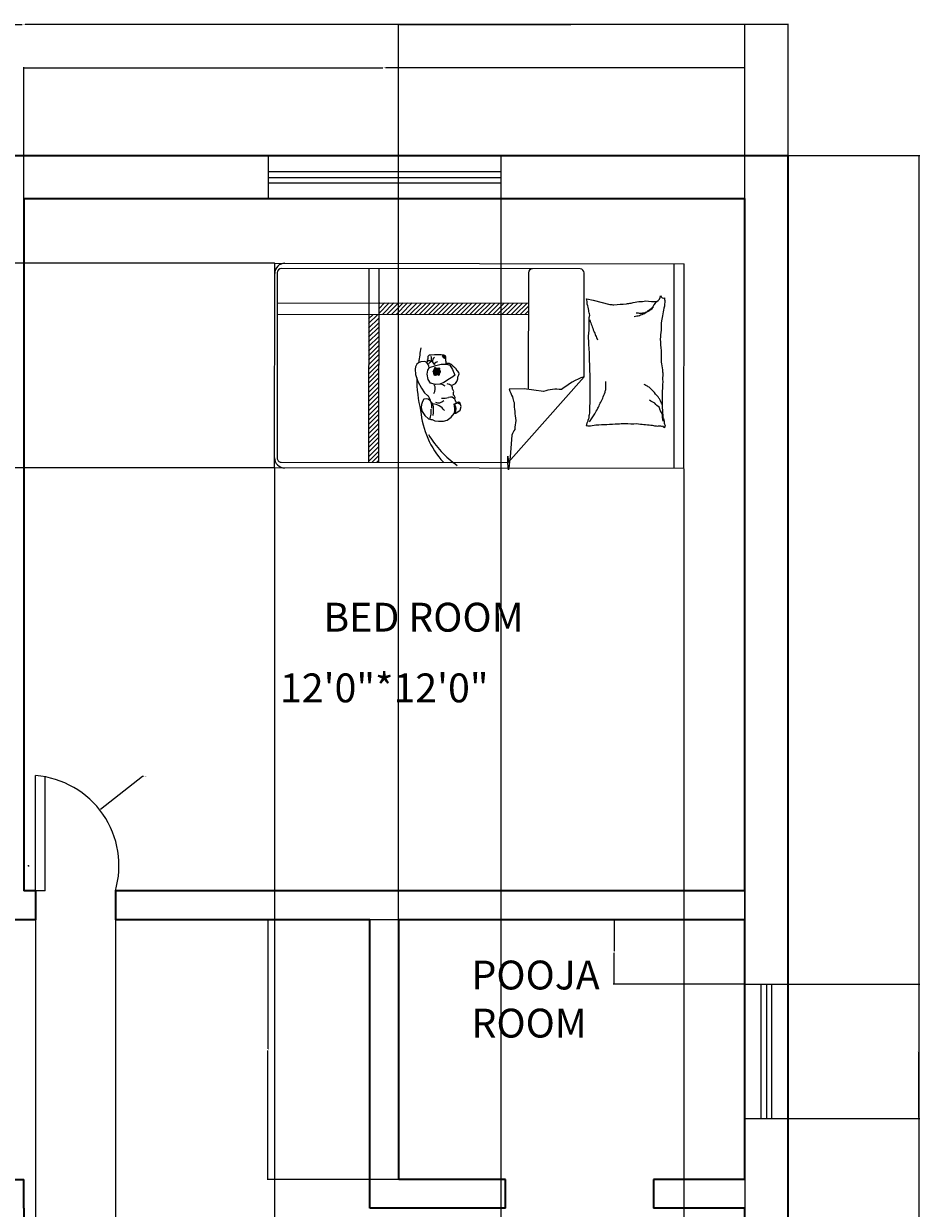
# Model space of a CAD drawing. Units: inches. Extents: x -17 to 1735, y -531 to 60.
# Tile 4 of 27: x 170 to 357, y -187 to 60. Entities that reach past the tile are written whole.
import ezdxf

# ---------------------------------------------------------------- set-up
doc = ezdxf.new("R2010")
doc.units = ezdxf.units.IN
doc.header["$MEASUREMENT"] = 0
for name, color, linetype, lineweight in [('A-ANNO-DIMS', 2, 'Continuous', 18), ('A-AREA-IDEN', 7, 'Continuous', 25), ('A-DOOR', 4, 'Continuous', 18), ('A-GLAZ', 4, 'Continuous', 18), ('A-WALL', 7, 'Continuous', 35)]:
    doc.layers.add(name, color=color, linetype=linetype, lineweight=lineweight)
doc.layers.add('A-FURN', color=242, linetype='Continuous', lineweight=18, true_color=0xcd2027)
doc.layers.add('A-FURN-PATT', color=242, linetype='Continuous', lineweight=13, true_color=0xcd2027)
doc.styles.get("Standard").update_dxf_attribs({"font": 'arial.ttf'})
doc.dimstyles.get("Standard").update_dxf_attribs({"dimtxt": 0.18, "dimasz": 0.18, "dimexe": 0.18, "dimexo": 0.0625, "dimgap": 0.09, "dimtad": 0, "dimtih": 1, "dimtoh": 1, "dimdec": 4, "dimzin": 0, "dimdsep": 46, "dimtxsty": 'Standard', "dimcen": 0.09, "dimadec": 0, "dimazin": 0, "dimtfac": 1, "dimtdec": 4, "dimtofl": 0, "dimtmove": 0, "dimatfit": 3, "dimfxl": 1, "dimtolj": 1, "dimtzin": 0, "dimarcsym": 0})
pattern_1 = [(314.93283, (734.16654, -492.2216), (0.082070428, 0.081878224), [])]

# ---------------------------------------------------------------- blocks, each defined once
blk = doc.blocks.new('WIN-FRAME-48IN')
for p, q in [((3.31, 48.33), (3.31, 0)), ((5.59, 0), (5.59, 48.33))]:
    blk.add_line(p, q)
blk.add_lwpolyline([(0, 48.33), (9, 48.33), (9, 0), (0, 0)], close=True)
blk = doc.blocks.new('*D9')
at = {"layer": 'A-ANNO-DIMS', "color": 0, "lineweight": -2, "transparency": 16777216}
for p, q in [((11.06, 32.29), (11.06, 59.62)), ((11.24, 59.44), (169.77, 59.44)), ((328.88, 59.44), (170.35, 59.44)), ((329.06, 32.29), (329.06, 59.62))]:
    blk.add_line(p, q, dxfattribs=at)
at = {"layer": 'A-ANNO-DIMS', "color": 0, "transparency": 16777216}
for points in [[(11.24, 59.47), (11.24, 59.41), (11.06, 59.44)], [(328.88, 59.47), (328.88, 59.41), (329.06, 59.44)]]:
    blk.add_solid(points, dxfattribs=at)
at = {"layer": 'Defpoints', "color": 0, "transparency": 16777216}
for p in [(329.06, 59.44), (11.06, 32.23), (329.06, 32.23)]:
    blk.add_point(p, dxfattribs=at)
at = {"layer": 'A-ANNO-DIMS', "color": 0, "transparency": 16777216, "insert": (170.06, 59.44), "char_height": 0.18, "attachment_point": 5}
blk.add_mtext('\\A1;318', dxfattribs=at)
blk = doc.blocks.new('*D10')
at = {"layer": 'A-ANNO-DIMS', "color": 0, "lineweight": -2, "transparency": 16777216}
for p, q in [((329.12, 32.23), (356.44, 32.23)), ((356.26, 32.05), (356.26, -235.74)), ((356.26, -503.9), (356.26, -236.11)), ((329.12, -504.08), (356.44, -504.08))]:
    blk.add_line(p, q, dxfattribs=at)
at = {"layer": 'A-ANNO-DIMS', "color": 0, "transparency": 16777216}
for points in [[(356.23, 32.05), (356.29, 32.05), (356.26, 32.23)], [(356.23, -503.9), (356.29, -503.9), (356.26, -504.08)]]:
    blk.add_solid(points, dxfattribs=at)
at = {"layer": 'Defpoints', "color": 0, "transparency": 16777216}
for p in [(329.06, 32.23), (329.06, -504.08), (356.26, -504.08)]:
    blk.add_point(p, dxfattribs=at)
at = {"layer": 'A-ANNO-DIMS', "color": 0, "transparency": 16777216, "insert": (356.26, -235.92), "char_height": 0.18, "attachment_point": 5}
blk.add_mtext('\\A1;536.3', dxfattribs=at)
blk = doc.blocks.new('*D12')
at = {"layer": 'A-ANNO-DIMS', "color": 0, "lineweight": -2, "transparency": 16777216}
for p, q in [((269.33, 23.18), (269.33, -531.46)), ((320.06, 23.17), (320.06, -531.46)), ((269.51, -531.28), (294.3, -531.28)), ((319.88, -531.28), (295.09, -531.28))]:
    blk.add_line(p, q, dxfattribs=at)
at = {"layer": 'A-ANNO-DIMS', "color": 0, "transparency": 16777216}
for points in [[(269.51, -531.25), (269.51, -531.31), (269.33, -531.28)], [(319.88, -531.25), (319.88, -531.31), (320.06, -531.28)]]:
    blk.add_solid(points, dxfattribs=at)
at = {"layer": 'Defpoints', "color": 0, "transparency": 16777216}
for p in [(269.33, 23.24), (320.06, 23.23), (320.06, -531.28)]:
    blk.add_point(p, dxfattribs=at)
at = {"layer": 'A-ANNO-DIMS', "color": 0, "transparency": 16777216, "insert": (294.7, -531.28), "char_height": 0.18, "attachment_point": 5}
blk.add_mtext('\\A1;50.73', dxfattribs=at)
blk = doc.blocks.new('*D18')
at = {"layer": 'A-ANNO-DIMS', "color": 0, "lineweight": -2, "transparency": 16777216}
for p, q in [((320, -126.77), (292.68, -126.77)), ((292.86, -126.95), (292.86, -133.29)), ((292.86, -139.99), (292.86, -133.65)), ((320, -140.17), (292.68, -140.17))]:
    blk.add_line(p, q, dxfattribs=at)
at = {"layer": 'A-ANNO-DIMS', "color": 0, "transparency": 16777216}
for points in [[(292.83, -126.95), (292.89, -126.95), (292.86, -126.77)], [(292.83, -139.99), (292.89, -139.99), (292.86, -140.17)]]:
    blk.add_solid(points, dxfattribs=at)
at = {"layer": 'Defpoints', "color": 0, "transparency": 16777216}
for p in [(292.86, -126.77), (320.06, -126.77), (320.06, -140.17)]:
    blk.add_point(p, dxfattribs=at)
at = {"layer": 'A-ANNO-DIMS', "color": 0, "transparency": 16777216, "insert": (292.86, -133.47), "char_height": 0.18, "attachment_point": 5}
blk.add_mtext('\\A1;13.4', dxfattribs=at)
blk = doc.blocks.new('*D19')
at = {"layer": 'A-ANNO-DIMS', "color": 0, "lineweight": -2, "transparency": 16777216}
for p, q in [((320.12, -140.17), (356.44, -140.17)), ((356.26, -140.35), (356.26, -153.94)), ((356.26, -167.9), (356.26, -154.31)), ((320.12, -168.08), (356.44, -168.08))]:
    blk.add_line(p, q, dxfattribs=at)
at = {"layer": 'A-ANNO-DIMS', "color": 0, "transparency": 16777216}
for points in [[(356.23, -140.35), (356.29, -140.35), (356.26, -140.17)], [(356.23, -167.9), (356.29, -167.9), (356.26, -168.08)]]:
    blk.add_solid(points, dxfattribs=at)
at = {"layer": 'Defpoints', "color": 0, "transparency": 16777216}
for p in [(320.06, -140.17), (320.06, -168.08), (356.26, -168.08)]:
    blk.add_point(p, dxfattribs=at)
at = {"layer": 'A-ANNO-DIMS', "color": 0, "transparency": 16777216, "insert": (356.26, -154.12), "char_height": 0.18, "attachment_point": 5}
blk.add_mtext('\\A1;27.91', dxfattribs=at)
blk = doc.blocks.new('*D25')
at = {"layer": 'A-ANNO-DIMS', "color": 0, "lineweight": -2, "transparency": 16777216}
for p, q in [((248.06, -126.71), (248.06, 59.62)), ((248.24, 59.44), (283.84, 59.44)), ((319.88, 59.44), (284.28, 59.44)), ((320.06, -126.71), (320.06, 59.62))]:
    blk.add_line(p, q, dxfattribs=at)
at = {"layer": 'A-ANNO-DIMS', "color": 0, "transparency": 16777216}
for points in [[(248.24, 59.47), (248.24, 59.41), (248.06, 59.44)], [(319.88, 59.47), (319.88, 59.41), (320.06, 59.44)]]:
    blk.add_solid(points, dxfattribs=at)
at = {"layer": 'Defpoints', "color": 0, "transparency": 16777216}
for p in [(320.06, 59.44), (248.06, -126.77), (320.06, -126.77)]:
    blk.add_point(p, dxfattribs=at)
at = {"layer": 'A-ANNO-DIMS', "color": 0, "transparency": 16777216, "insert": (284.06, 59.44), "char_height": 0.18, "attachment_point": 5}
blk.add_mtext('\\A1;72', dxfattribs=at)
blk = doc.blocks.new('*D26')
at = {"layer": 'A-ANNO-DIMS', "color": 0, "lineweight": -2, "transparency": 16777216}
for p, q in [((248, -126.77), (220.68, -126.77)), ((220.86, -126.95), (220.86, -153.59)), ((220.86, -180.59), (220.86, -153.95)), ((248, -180.77), (220.68, -180.77))]:
    blk.add_line(p, q, dxfattribs=at)
at = {"layer": 'A-ANNO-DIMS', "color": 0, "transparency": 16777216}
for points in [[(220.83, -126.95), (220.89, -126.95), (220.86, -126.77)], [(220.83, -180.59), (220.89, -180.59), (220.86, -180.77)]]:
    blk.add_solid(points, dxfattribs=at)
at = {"layer": 'Defpoints', "color": 0, "transparency": 16777216}
for p in [(220.86, -126.77), (248.06, -126.77), (248.06, -180.77)]:
    blk.add_point(p, dxfattribs=at)
at = {"layer": 'A-ANNO-DIMS', "color": 0, "transparency": 16777216, "insert": (220.86, -153.77), "char_height": 0.18, "attachment_point": 5}
blk.add_mtext('\\A1;54', dxfattribs=at)
blk = doc.blocks.new('*D31')
at = {"layer": 'A-ANNO-DIMS', "color": 0, "lineweight": -2, "transparency": 16777216}
for p, q in [((172.55, -126.83), (172.55, -531.46)), ((189.13, -126.83), (189.13, -531.46)), ((172.73, -531.28), (180.46, -531.28)), ((188.95, -531.28), (181.23, -531.28))]:
    blk.add_line(p, q, dxfattribs=at)
at = {"layer": 'A-ANNO-DIMS', "color": 0, "transparency": 16777216}
for points in [[(172.73, -531.25), (172.73, -531.31), (172.55, -531.28)], [(188.95, -531.25), (188.95, -531.31), (189.13, -531.28)]]:
    blk.add_solid(points, dxfattribs=at)
at = {"layer": 'Defpoints', "color": 0, "transparency": 16777216}
for p in [(172.55, -126.77), (189.13, -126.77), (189.13, -531.28)]:
    blk.add_point(p, dxfattribs=at)
at = {"layer": 'A-ANNO-DIMS', "color": 0, "transparency": 16777216, "insert": (180.84, -531.28), "char_height": 0.18, "attachment_point": 5}
blk.add_mtext('\\A1;16.58', dxfattribs=at)
blk = doc.blocks.new('*D37')
at = {"layer": 'A-ANNO-DIMS', "color": 0, "lineweight": -2, "transparency": 16777216}
for p, q in [((222.24, -32.84), (222.24, -531.46)), ((307.4, -32.94), (307.4, -531.46)), ((222.42, -531.28), (264.43, -531.28)), ((307.22, -531.28), (265.21, -531.28))]:
    blk.add_line(p, q, dxfattribs=at)
at = {"layer": 'A-ANNO-DIMS', "color": 0, "transparency": 16777216}
for points in [[(222.42, -531.25), (222.42, -531.31), (222.24, -531.28)], [(307.22, -531.25), (307.22, -531.31), (307.4, -531.28)]]:
    blk.add_solid(points, dxfattribs=at)
at = {"layer": 'Defpoints', "color": 0, "transparency": 16777216}
for p in [(222.24, -32.78), (307.4, -32.88), (307.4, -531.28)]:
    blk.add_point(p, dxfattribs=at)
at = {"layer": 'A-ANNO-DIMS', "color": 0, "transparency": 16777216, "insert": (264.82, -531.28), "char_height": 0.18, "attachment_point": 5}
blk.add_mtext('\\A1;85.16', dxfattribs=at)
blk = doc.blocks.new('*D38')
at = {"layer": 'A-ANNO-DIMS', "color": 0, "lineweight": -2, "transparency": 16777216}
for p, q in [((222.23, 9.8), (-16.4, 9.8)), ((-16.22, 9.62), (-16.22, -11.31)), ((-16.22, -32.6), (-16.22, -11.67)), ((222.18, -32.78), (-16.4, -32.78))]:
    blk.add_line(p, q, dxfattribs=at)
at = {"layer": 'A-ANNO-DIMS', "color": 0, "transparency": 16777216}
for points in [[(-16.25, 9.62), (-16.19, 9.62), (-16.22, 9.8)], [(-16.25, -32.6), (-16.19, -32.6), (-16.22, -32.78)]]:
    blk.add_solid(points, dxfattribs=at)
at = {"layer": 'Defpoints', "color": 0, "transparency": 16777216}
for p in [(222.29, 9.8), (-16.22, -32.78), (222.24, -32.78)]:
    blk.add_point(p, dxfattribs=at)
at = {"layer": 'A-ANNO-DIMS', "color": 0, "transparency": 16777216, "insert": (-16.22, -11.49), "char_height": 0.18, "attachment_point": 5}
blk.add_mtext('\\A1;42.58', dxfattribs=at)
blk = doc.blocks.new('*D43')
at = {"layer": 'A-ANNO-DIMS', "color": 0, "lineweight": -2, "transparency": 16777216}
for p, q in [((170.06, 23.29), (170.06, 50.61)), ((170.24, 50.43), (244.78, 50.43)), ((319.88, 50.43), (245.34, 50.43)), ((320.06, 23.29), (320.06, 50.61))]:
    blk.add_line(p, q, dxfattribs=at)
at = {"layer": 'A-ANNO-DIMS', "color": 0, "transparency": 16777216}
for points in [[(170.24, 50.46), (170.24, 50.4), (170.06, 50.43)], [(319.88, 50.46), (319.88, 50.4), (320.06, 50.43)]]:
    blk.add_solid(points, dxfattribs=at)
at = {"layer": 'Defpoints', "color": 0, "transparency": 16777216}
for p in [(320.06, 50.43), (170.06, 23.23), (320.06, 23.23)]:
    blk.add_point(p, dxfattribs=at)
at = {"layer": 'A-ANNO-DIMS', "color": 0, "transparency": 16777216, "insert": (245.06, 50.43), "char_height": 0.18, "attachment_point": 5}
blk.add_mtext('\\A1;150', dxfattribs=at)
blk = doc.blocks.new('*D54')
at = {"layer": 'A-ANNO-DIMS', "color": 0, "lineweight": -2, "transparency": 16777216}
for p, q in [((194.79, -96.99), (186.04, -103.83)), ((194.97, -96.99), (194.79, -96.99)), ((170.99, -115.51), (171.17, -115.51)), ((171.08, -115.6), (171.08, -115.42))]:
    blk.add_line(p, q, dxfattribs=at)
at = {"layer": 'A-ANNO-DIMS', "color": 0, "transparency": 16777216}
blk.add_solid([(186.02, -103.8), (186.06, -103.85), (185.9, -103.94)], dxfattribs=at)
at = {"layer": 'Defpoints', "color": 0, "transparency": 16777216}
for p in [(185.9, -103.94), (171.08, -115.51)]:
    blk.add_point(p, dxfattribs=at)
at = {"layer": 'A-ANNO-DIMS', "color": 0, "transparency": 16777216, "insert": (195.38, -96.99), "char_height": 0.18, "attachment_point": 5}
blk.add_mtext('\\A1;R18.8', dxfattribs=at)

msp = doc.modelspace()

# ---------------------------------------------------------------- hatches: boundary and pattern name
at = {"layer": 'A-FURN-PATT'}
h = msp.add_hatch(dxfattribs=at)
h.set_pattern_fill('ANSI31', color=256, scale=0.21291, angle=-90.06717, style=0)
h.set_pattern_definition([(44.9328, (336.72006, -40.7893), (0.477435, -0.4785558), [])])
h.paths.add_polyline_path([(243.9098, 1.5357), (243.907, -0.8463), (275.0288, -0.8828), (275.0316, 1.4992)])
h.paths.add_polyline_path([(241.8205, -0.8439), (241.7845, -31.5931), (243.871, -31.5955), (243.907, -0.8463)])
h = msp.add_hatch(dxfattribs=at)
h.set_pattern_fill('ANSI31', color=256, scale=0.927434, angle=-90.06717, style=0)
h.set_pattern_definition(pattern_1)
h.paths.add_polyline_path([(257.8751, -9.9217), (257.8615, -9.709), (257.7919, -9.5225), (257.6134, -9.3824), (257.4737, -9.3201), (257.1071, -9.2829, 0.47935676)])
h = msp.add_hatch(dxfattribs=at)
h.set_pattern_fill('ANSI31', color=256, scale=0.927434, angle=-90.06717, style=0)
h.set_pattern_definition(pattern_1)
h.paths.add_polyline_path([(255.3459, -12.9354), (255.3281, -13.1639), (255.4098, -13.3866), (255.5619, -13.5157), (255.7375, -13.5159), (255.9894, -13.399), (256.1769, -13.3582), (256.2646, -13.4286), (256.3816, -13.4873), (256.5222, -13.4289), (256.5458, -13.3176), (256.5518, -13.1887), (256.6047, -13.0189), (256.7455, -12.8023), (256.769, -12.7437), (256.6229, -12.4916), (256.582, -12.3802), (256.6115, -12.2045), (256.6292, -12.0815), (256.5181, -11.9642), (256.4009, -12.005), (256.3013, -12.1221), (256.0846, -12.0984), (255.7042, -11.9456), (255.5227, -11.9806), (255.4991, -12.1036), (255.4756, -12.1973), (255.376, -12.2733), (255.3817, -12.3671), (255.3288, -12.5252), (255.2233, -12.6364), (255.1705, -12.6949), (255.2583, -12.7654)])

# ---------------------------------------------------------------- linework, layer by layer
at = {"layer": 'A-DOOR'}
for p, q in [((172.5508, -120.7685), (172.5508, -96.7685)), ((174.5508, -120.7685), (174.5508, -97.0339)), ((174.5508, -120.7685), (172.5508, -120.7685))]:
    msp.add_line(p, q, dxfattribs=at)
msp.add_arc((171.0813, -115.5103), 18.7993, 343.75767, 85.516486, dxfattribs=at)
at = {"layer": 'A-FURN'}
for p, q in [((222.238, -32.7807), (222.2879, 9.8012)), ((222.2879, 9.8012), (307.4519, 9.7014)), ((222.8038, 7.8496), (222.7586, -30.7191)), ((285.7962, 8.6274), (223.6564, 8.7003)), ((241.8317, 8.679), (241.7845, -31.5931)), ((243.9182, 8.6765), (243.871, -31.5955)), ((275.039, 7.7884), (275.0106, -16.4244)), ((286.6215, -13.8065), (286.6468, 7.7748)), ((286.6215, -13.8065), (270.8545, -31.6271)), ((223.6092, -31.5717), (270.8545, -31.6271)), ((307.402, -32.8805), (222.238, -32.7807))]:
    msp.add_line(p, q, dxfattribs=at)
for points in [[(305.3228, 9.7039), (305.2729, -32.878)], [(307.402, -32.8805), (307.4519, 9.7014)], [(222.7964, 1.5604), (275.0316, 1.4992)], [(222.7936, -0.8216), (275.0288, -0.8828)], [(256.7756, -9.2714), (256.2062, -9.2442), (255.544, -9.2832), (254.8421, -9.3089), (254.6302, -9.3351), (254.3786, -9.3481), (254.1134, -9.626), (254.0998, -9.8911), (254.1526, -10.0899), (254.0199, -10.2885), (254.0727, -10.4741), (253.9266, -10.8185), (253.7544, -10.7918), (253.5162, -10.659), (252.6686, -10.6845), (252.1784, -10.9357), (251.8734, -11.2004), (251.5418, -11.7168), (251.4617, -12.26), (251.5796, -13.3203), (252.0679, -14.8183), (252.8079, -16.1576), (253.4291, -17.1654), (254.0774, -17.7095), (254.223, -17.8157), (254.6326, -18.6112), (254.6457, -18.6908), (254.5662, -18.7702), (254.1692, -18.5047), (253.8779, -18.4248), (253.3084, -18.4904), (253.0033, -18.9406), (252.8017, -19.5555), (252.7722, -20.3004), (252.9717, -21.0455), (253.5147, -21.8769), (254.2869, -22.5367), (254.7448, -22.7091), (255.0024, -22.7381), (255.5748, -22.9679), (256.3476, -23.0834), (257.3783, -23.0846), (258.1802, -22.8564), (258.9826, -22.2271), (259.5847, -21.4543), (259.9856, -21.3688), (260.8739, -20.7396), (261.0752, -19.9663), (260.7612, -19.1352), (260.475, -19.0775), (260.191, -19.3182), (260.1092, -19.3415), (259.9928, -19.061), (259.8997, -18.874), (259.853, -18.8272), (259.8066, -18.5818), (259.7483, -18.5), (259.7955, -18.1029), (259.6092, -17.7289), (259.4809, -17.6119), (259.4698, -17.1096), (259.5284, -16.8877), (259.3422, -16.4553), (259.2605, -16.4085), (259.2259, -16.0113), (259.0628, -15.7307), (259.1564, -15.5439), (259.4368, -15.4041), (259.8806, -15.1827), (260.1846, -14.8326), (260.2784, -14.4589), (260.3487, -14.2487), (260.3724, -13.9217), (260.4194, -13.6764), (260.5598, -13.3846), (260.6184, -13.2211), (260.607, -12.929), (260.3156, -12.5666), (260.1523, -12.5197), (260.0126, -12.1924), (259.8844, -12.0054), (259.721, -11.9468), (259.6394, -11.8532), (259.5695, -11.748), (259.3245, -11.6309), (259.2661, -11.5841), (259.2662, -11.5024), (259.033, -11.2801), (258.9281, -11.1749), (258.7413, -11.1863), (258.5547, -11.0343), (258.3912, -11.0458), (258.0878, -11.022), (257.9477, -10.9868), (257.8911, -10.9522), (257.9145, -10.8823), (257.9303, -10.6803), (257.8528, -10.5248), (257.8451, -10.4394), (257.8844, -10.0665), (257.8615, -9.709), (257.7919, -9.5225), (257.6134, -9.3824), (257.4737, -9.3201), (256.9303, -9.265), (256.7756, -9.2714)], [(258.7068, -11.3756), (259.2271, -12.3079), (259.71, -13.4638), (259.3185, -13.8361), (258.6476, -14.2452), (257.4735, -14.9892), (256.6351, -15.3237), (255.7411, -15.4158), (254.6986, -15.1537), (254.2153, -14.3891), (254.0117, -13.2894), (254.1058, -12.4696), (254.4417, -11.8737), (255.8202, -11.4654), (256.9192, -11.2244), (258.0739, -11.1885), (258.7068, -11.3756)], [(256.769, -12.7437), (256.6229, -12.4916), (256.582, -12.3802), (256.6115, -12.2045), (256.6292, -12.0815), (256.5181, -11.9642), (256.4009, -12.005), (256.3013, -12.1221), (256.0846, -12.0984), (255.7042, -11.9456), (255.5227, -11.9806), (255.4991, -12.1036), (255.4756, -12.1973), (255.376, -12.2733), (255.3817, -12.3671), (255.3288, -12.5252), (255.2233, -12.6364), (255.1705, -12.6949), (255.2583, -12.7654), (255.3459, -12.9354), (255.3281, -13.1639), (255.4098, -13.3866), (255.5619, -13.5157), (255.7375, -13.5159), (255.9894, -13.399), (256.1769, -13.3582), (256.2646, -13.4286), (256.3816, -13.4873), (256.5222, -13.4289), (256.5458, -13.3176), (256.5518, -13.1887), (256.6047, -13.0189), (256.7455, -12.8023), (256.769, -12.7437)]]:
    msp.add_lwpolyline(points, dxfattribs=at)
for points in [[(301.7532, 1.827, 0.26336794), (302.5546, 3.0163, 0.49481805), (303.3523, 2.6248, 0.04922472), (303.4257, 1.8722, 0.03683084), (303.3502, 0.8656, 0.03189269), (303.0019, -0.7512, -0.035782), (302.7026, -2.195, -0.03294126), (302.4463, -6.0126, -0.02656446), (302.6926, -10.7492, -0.01790542), (302.9191, -12.3469, 0.03339746), (303.0141, -13.2075, 0.03203963), (302.981, -14.7865, -0.01844195), (302.8492, -17.5253, -0.01083729), (302.878, -20.2831, -0.01462385), (303.0034, -22.3232, -0.11124937), (303.3134, -23.2837, 0.15370834), (303.4809, -24.003, 0.07644442), (303.4071, -24.3196, 0.21551229), (303.3206, -24.4027, 0.58585823), (303.1911, -24.2891, -0.36348931), (303.0812, -24.0825, -0.19171627), (302.5901, -24.0795, 0.1296753), (301.8825, -24.1611, 0.01735021), (301.1671, -24.0325, -0.01932565), (300.5243, -23.9196, -0.01881752), (297.6128, -23.6345, -0.0218281), (295.0909, -23.5934, -0.00620415), (293.6494, -23.6507, -0.00196306), (289.0974, -23.9062, -0.02834083), (287.5587, -24.0865, 0.11701353), (287.1794, -24.0639, 0.36605999), (287.1398, -24.003, 0.03973043), (287.26, -23.4243, 0.04830882), (287.4941, -22.8395, -0.06298072), (287.6608, -22.3852, -0.04057963), (287.8059, -21.3891, -0.01434509), (287.905, -18.5473, -0.00548442), (287.8794, -13.2056, -0.00715271), (287.7563, -9.1115, -0.00876157), (287.644, -7.2997, 0.00815313), (287.5209, -5.3529, 0.06251003), (287.7112, -2.9205, -0.07866929), (287.8003, -0.9794, -0.04782509), (287.6006, -0.027, 0.03449399), (287.289, 1.2843, 0.02357139), (287.1619, 2.3632, 0.51022848), (287.2104, 2.4038), (288.4886, 2.0825), (292.0035, 1.1988, -0.07304094), (292.8372, 1.1147, -0.0233051), (295.4398, 1.3547, -0.01829889), (296.4128, 1.5268, 0.01096989), (298.031, 1.8377, 0.04228119), (299.4923, 1.9598, 0.02720053), (301.7658, 1.8333)], [(301.7538, 1.8346, 0.07737943), (300.673, 0.3536, 0.07737943), (299.1931, -0.7288, 0.04752549), (298.1443, -1.1502, 0.04752549), (297.0348, -1.366)], [(301.0699, 0.7077, 0.05368995), (300.5166, 0.1034, 0.07031175), (299.9927, -0.2411, 0.01544823), (299.6283, -0.3997, 0.01324357), (299.1933, -0.56, 0.08212667), (298.4232, -0.6865, 0.0641637), (297.4353, -0.558)], [(287.8295, -2.0056, -0.00972947), (288.2127, -3.1681, -0.00972947), (288.6409, -4.3147, -0.0079705), (289.0247, -5.2411, -0.0079705), (289.4378, -6.1548)], [(286.6215, -13.8065, 0.08527182), (281.9298, -16.4967, 0.12404448), (278.2022, -16.8845), (274.1402, -16.2989), (271.0518, -16.3697)], [(271.0518, -16.3697, 0.02736216), (271.7497, -18.0127, 0.04083428), (272.0637, -19.1681, 0.03844124), (272.4642, -22.9002, 0.07652788), (272.2324, -24.7797, 0.10364867), (271.6198, -25.9505, -0.01877781), (270.9082, -33.1946, -0.02403749), (270.7501, -30.3049, -0.05231485), (270.8545, -31.6271)], [(287.7398, -23.1761, -0.01610775), (288.8587, -21.5202, -0.02459883), (289.5011, -20.3795, -0.00947722), (290.4956, -18.2925, -0.01593728), (291.0233, -17.0228, -0.07252085), (291.1768, -16.3272, -0.03333928), (291.1857, -14.7841)], [(302.8439, -19.5428, -0.02784216), (302.3932, -18.5296, -0.04868501), (302.0496, -17.9953, -0.02366646), (301.0137, -16.8051, -0.03122342), (300.1341, -15.994, -0.04680097), (299.8079, -15.7761, -0.02319083), (299.0959, -15.433)], [(303.0825, -23.0342, -0.08815313), (302.9333, -21.5637, -0.08815313), (302.2867, -20.2345, -0.07754712), (301.3675, -19.3117, -0.07754712), (300.2108, -18.7128)]]:
    msp.add_lwpolyline(points, format="xyb", dxfattribs=at)
for centre, radius, start, end in [((224.4145, 7.6696), 2.1291, 89.93283, 179.93283), ((223.6555, 7.8486), 0.8516, 89.93283, 179.93283), ((275.8906, 7.7874), 0.8516, 89.93283, 179.93283), ((285.7952, 7.7758), 0.8516, 359.93283, 89.93283), ((294.6673, -15.5175), 42.688, 169.554494, 173.680063), ((253.0659, -10.1049), 1.8186, 344.775022, 17.172556), ((256.2738, -10.6408), 1.1772, 129.677913, 181.666549), ((257.7477, -9.2938), 0.6407, 179.03157, 281.475749), ((252.9689, -11.9612), 1.4088, 2.082591, 56.11115), ((254.4896, -11.027), 0.5384, 86.132249, 138.999385), ((255.0093, -11.5015), 0.7913, 115.147666, 159.73395), ((253.9879, -12.2975), 1.886, 30.521411, 73.424064), ((256.3057, -11.5998), 0.9188, 99.893336, 151.775863), ((279.8743, -14.2019), 28.0509, 179.729027, 193.694468), ((253.8487, -16.3206), 1.8124, 327.447786, 27.168441), ((256.5334, -17.0594), 1.7387, 46.72769, 86.648422), ((256.3989, -21.524), 6.4808, 65.274281, 74.424089), ((256.3785, -17.9657), 1.9305, 203.339128, 230.823738), ((251.9477, -19.9986), 3.0185, 352.902018, 16.73158), ((249.5013, -20.924), 5.8435, 350.941245, 14.486866), ((254.8902, -22.7583), 3.3071, 35.854778, 85.338343), ((256.2994, -17.6668), 1.5876, 247.361471, 315.96913), ((257.0236, -12.5551), 5.7189, 269.217609, 284.441708), ((258.8147, -19.2046), 1.1697, 37.040849, 108.176353), ((259.6322, -18.8909), 0.5631, 263.887014, 320.950793), ((258.2847, -20.5826), 1.7142, 331.081844, 41.316461), ((256.8401, -20.4697), 2.9159, 340.264742, 20.450947), ((260.172, -19.9675), 0.6833, 38.235952, 78.870253), ((271.2455, -19.0833), 18.7076, 185.396918, 222.042012), ((250.3197, -20.8948), 4.5381, 337.616569, 4.523041), ((273.3022, -14.0829), 22.3831, 211.703622, 234.270288), ((224.3696, -30.6563), 2.1291, 179.93283, 269.93283), ((223.6102, -30.7201), 0.8516, 179.93283, 269.93283)]:
    msp.add_arc(centre, radius, start, end, dxfattribs=at)
at = {"layer": 'A-GLAZ'}
for p, q in [((221.0072, 27.6142), (269.333, 27.6142)), ((323.3729, -140.1683), (323.3729, -168.0787)), ((324.5903, -140.1683), (324.5903, -168.0787)), ((325.6545, -168.0787), (325.6545, -140.1683)), ((320.0618, -168.0787), (329.0618, -168.0787))]:
    msp.add_line(p, q, dxfattribs=at)
msp.add_lwpolyline([(320.0618, -168.0787), (320.0618, -140.1683), (329.0618, -140.1683), (329.0618, -168.0787)], dxfattribs=at)
at = {"layer": 'A-WALL'}
for p, q in [((11.0618, 32.2315), (320.0618, 32.2315)), ((320.0618, 32.2315), (329.0618, 32.2315)), ((329.0618, -495.0795), (329.0618, 32.2315)), ((170.0618, 23.2315), (170.0618, -120.7685)), ((170.0618, 23.2315), (320.0618, 23.2315)), ((320.0618, -120.7685), (320.0618, 23.2315)), ((172.5508, -120.7685), (170.0618, -120.7685)), ((172.5508, -120.7685), (172.5508, -126.7685)), ((320.0618, -120.7685), (189.1303, -120.7685)), ((189.1303, -120.7685), (189.1303, -126.7685)), ((172.5508, -126.7685), (161.9382, -126.7685)), ((242.0618, -126.7685), (189.1303, -126.7685)), ((242.0618, -186.7685), (242.0618, -126.7685)), ((320.0618, -126.7685), (248.0618, -126.7685)), ((248.0618, -180.7685), (248.0618, -126.7685)), ((320.0618, -180.7685), (320.0618, -126.7685)), ((110.0618, -180.7685), (170.0618, -180.7685)), ((170.0618, -186.7685), (170.0618, -180.7685)), ((270.2983, -180.7685), (248.0618, -180.7685)), ((270.2983, -186.7685), (270.2983, -180.7685)), ((320.0618, -180.7685), (301.0793, -180.7685)), ((301.0793, -180.7685), (301.0793, -186.7685)), ((170.0618, -186.7685), (170.0618, -296.302)), ((248.0618, -186.7685), (242.0618, -186.7685)), ((270.2983, -186.7685), (248.0618, -186.7685)), ((320.0618, -186.7685), (301.0793, -186.7685)), ((320.0618, -495.0795), (320.0618, -186.7685))]:
    msp.add_line(p, q, dxfattribs=at)

# ---------------------------------------------------------------- block references
at = {"layer": 'A-GLAZ', "rotation": 89.99999999999991}
msp.add_blockref('WIN-FRAME-48IN', (269.3329, 23.241), dxfattribs=at)

# ---------------------------------------------------------------- texts
at = {"layer": 'A-ANNO-DIMS', "insert": (223.3605, -75.5272), "char_height": 6, "attachment_point": 1}
msp.add_mtext_dynamic_manual_height_columns('12\'0"*12\'0"', width=68.089628, gutter_width=1, heights=[0], dxfattribs=at)
at = {"layer": 'A-AREA-IDEN', "char_height": 6, "attachment_point": 1}
for s, width, insert in [('BED ROOM', 54.663685, (232.391, -60.8223)), ('POOJA ROOM', 48.503804, (263.2032, -135.2507))]:
    msp.add_mtext_dynamic_manual_height_columns(s, width=width, gutter_width=1, heights=[0], dxfattribs=dict(at, insert=insert))

# ---------------------------------------------------------------- dimensions: what is measured, and where the dimension line sits
at = {"layer": 'A-ANNO-DIMS'}
for base, p1, p2, override, picture, middle in [((329.0618, 59.4408), (11.0618, 32.2315), (329.0618, 32.2315), {"dimdec": 0, "dimlfac": 1, "dimrnd": 0, "dimzin": 0, "dimdsep": 46, "dimlunit": 2}, '*D9', (170.0618, 59.4408)), ((320.0618, 59.4408), (248.0618, -126.7685), (320.0618, -126.7685), {"dimdec": 0, "dimlfac": 1, "dimrnd": 0, "dimzin": 0, "dimdsep": 46, "dimlunit": 2}, '*D25', (284.0618, 59.4408)), ((320.0618, -531.2795), (269.333, 23.2408), (320.0618, 23.2315), {"dimdec": 2, "dimlfac": 1, "dimrnd": 0, "dimzin": 0, "dimdsep": 46, "dimlunit": 2}, '*D12', (294.6974, -531.2795)), ((307.402, -531.2795), (222.238, -32.7807), (307.402, -32.8805), {"dimdec": 2, "dimlfac": 1, "dimrnd": 0, "dimzin": 0, "dimdsep": 46, "dimlunit": 2}, '*D37', (264.82, -531.2795)), ((189.1303, -531.2795), (172.5508, -126.7685), (189.1303, -126.7685), {"dimdec": 2, "dimlfac": 1, "dimrnd": 0, "dimzin": 0, "dimdsep": 46, "dimlunit": 2}, '*D31', (180.8406, -531.2795))]:
    dim = msp.add_linear_dim(base=base, p1=p1, p2=p2, dimstyle='Standard', override=override, dxfattribs=at)
    dim.commit()
    dim.dimension.update_dxf_attribs({"geometry": picture, "text_midpoint": middle})
for base, p1, p2, angle, override, picture, middle in [((320.0618, 50.4315), (170.0618, 23.2315), (320.0618, 23.2315), 0, {"dimdec": 0, "dimlfac": 1, "dimrnd": 0, "dimzin": 0, "dimdsep": 46, "dimlunit": 2}, '*D43', (245.0618, 50.4315)), ((356.2618, -504.0795), (329.0618, 32.2315), (329.0618, -504.0795), 270, {"dimdec": 1, "dimlfac": 1, "dimrnd": 0, "dimzin": 0, "dimdsep": 46, "dimlunit": 2}, '*D10', (356.2618, -235.924)), ((-16.2237, -32.7807), (222.2879, 9.8012), (222.238, -32.7807), 90, {"dimdec": 2, "dimlfac": 1, "dimrnd": 0, "dimzin": 0, "dimdsep": 46, "dimlunit": 2}, '*D38', (-16.2237, -11.4897)), ((220.8618, -126.7685), (248.0618, -180.7685), (248.0618, -126.7685), 90, {"dimdec": 0, "dimlfac": 1, "dimrnd": 0, "dimzin": 0, "dimdsep": 46, "dimlunit": 2}, '*D26', (220.8618, -153.7685)), ((292.8618, -126.7685), (320.0618, -140.1683), (320.0618, -126.7685), 90, {"dimdec": 1, "dimlfac": 1, "dimrnd": 0, "dimzin": 0, "dimdsep": 46, "dimlunit": 2}, '*D18', (292.8618, -133.4684)), ((356.2618, -168.0787), (320.0618, -140.1683), (320.0618, -168.0787), 90, {"dimdec": 2, "dimlfac": 1, "dimrnd": 0, "dimzin": 0, "dimdsep": 46, "dimlunit": 2}, '*D19', (356.2618, -154.1235))]:
    dim = msp.add_linear_dim(base=base, p1=p1, p2=p2, angle=angle, dimstyle='Standard', override=override, dxfattribs=at)
    dim.commit()
    dim.dimension.update_dxf_attribs({"geometry": picture, "text_midpoint": middle})
dim = msp.add_radius_dim(center=(171.0813, -115.5103), mpoint=(185.8968, -103.9382), dimstyle='Standard', override={"dimdec": 1, "dimlfac": 1, "dimrnd": 0, "dimzin": 0, "dimdsep": 46, "dimlunit": 2}, dxfattribs=at)
dim.commit()
dim.dimension.update_dxf_attribs({"geometry": '*D54', "text_midpoint": (195.3763, -96.9949), "dimtype": 164})

doc.saveas('drawing.dxf')
